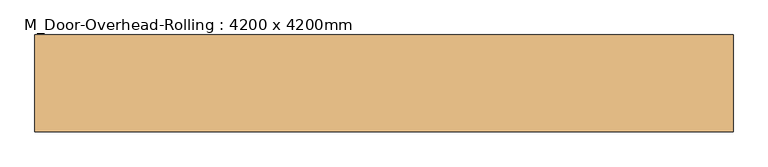
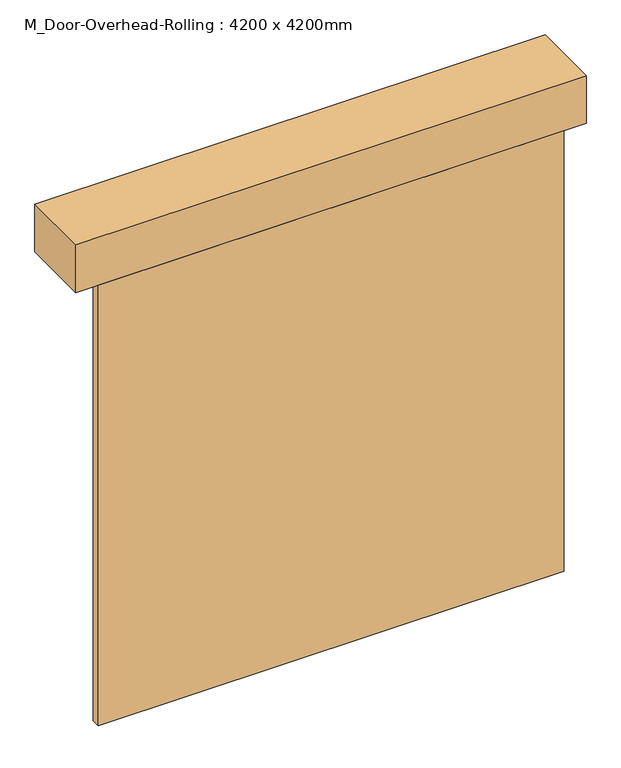
"""IFC4 building model written with IfcOpenShell, lengths in millimetres: door geometry, M_Door-Overhead-Rolling : 4200 x 4200mm."""

from ifc_helpers import new_model, si_unit, frame, origin, origin_with_axes, place, context, project, spatial, polyline, outline, extrude, source, transform, mapped, element, save


def m_door_overhead_rolling_4200_x_4200mm_f21f583b(model_context):
    return source(origin(), model_context, "Body", "SweptSolid", [
        extrude(outline(polyline([(2100.0, 114.3), (-2100.0, 114.3), (-2100.0, 194.3), (2100.0, 194.3), (2100.0, 114.3)])), origin_with_axes(), (0.0, 0.0, 1.0), 4200.0),
        extrude(outline(polyline([(2303.2, 753.1), (2303.2, 114.3), (-2303.2, 114.3), (-2303.2, 753.1), (2303.2, 753.1)])), frame((0.0, 0.0, 4200.0), z_axis=(0.0, 0.0, 1.0), x_axis=(1.0, 0.0, 0.0)), (0.0, 0.0, 1.0), 457.2),
    ])


if __name__ == "__main__":
    model = new_model("IFC4")
    model_context = context("Model", 3, world=origin())
    ifc_project = project(units=[si_unit("LENGTHUNIT", "METRE", prefix="MILLI")], contexts=[model_context])
    site = spatial("IfcSite", under=ifc_project)
    building = spatial("IfcBuilding", under=site)
    placement = place(None, origin())
    m_door_overhead_rolling_4200_x_4200mm_shape = m_door_overhead_rolling_4200_x_4200mm_f21f583b(model_context)
    element("IfcDoor", 1, ObjectType="M_Door-Overhead-Rolling : 4200 x 4200mm", at=placement, inside=building, context=model_context, shape_type="MappedRepresentation", body=[
        mapped(m_door_overhead_rolling_4200_x_4200mm_shape, transform((0.0, 0.0, 0.0), x_axis=(1.0, 0.0, 0.0), y_axis=(0.0, 1.0, 0.0), z_axis=(0.0, 0.0, 1.0))),
    ])
    save(model, "model.ifc")

# Revit data of these elements
# Type "M_Door-Overhead-Rolling : 4200 x 4200mm"
#   Type Mark = "40"
#   Construction Type Id = "MDOOR"
#   Assembly Code = "B2030400"
#   Analytic Construction = "Metal"
#   Thickness = 80 mm
#   Rough Width [instance default] = 4200 mm
#   Rough Height [instance default] = 4200 mm
#   Heat Transfer Coefficient (U) = 3.7021 W/(m²·K)
#   Height [instance default] = 4200 mm
#   Width [instance default] = 4200 mm
#   Define Thermal Properties by = 1
#   Function = 1
#   Roller Material = Steel, Paint Finish, Ivory, Matte
#   Roller Box Material = Steel, Paint Finish, Ivory, Matte
#   Visual Light Transmittance = 0
#   Solar Heat Gain Coefficient = 0
#   Wall Closure = (empty or 0)
# Element 1 (IfcDoor, "M_Door-Overhead-Rolling : 4200 x 4200mm")
#   Materials on its faces: "Steel, Paint Finish, Ivory, Matte"
# Materials
#   "Steel, Paint Finish, Ivory, Matte": class "Metal", colour RGB 247 247 239, transparency 0, Description = "Steel, paint finish, ivory, matte", Cost = 0
